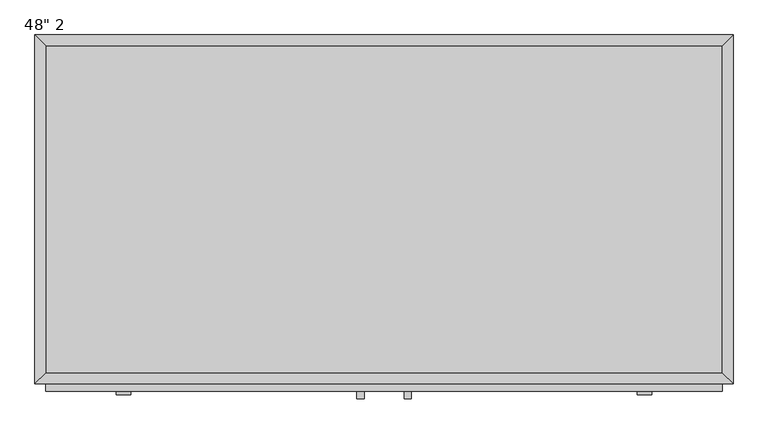
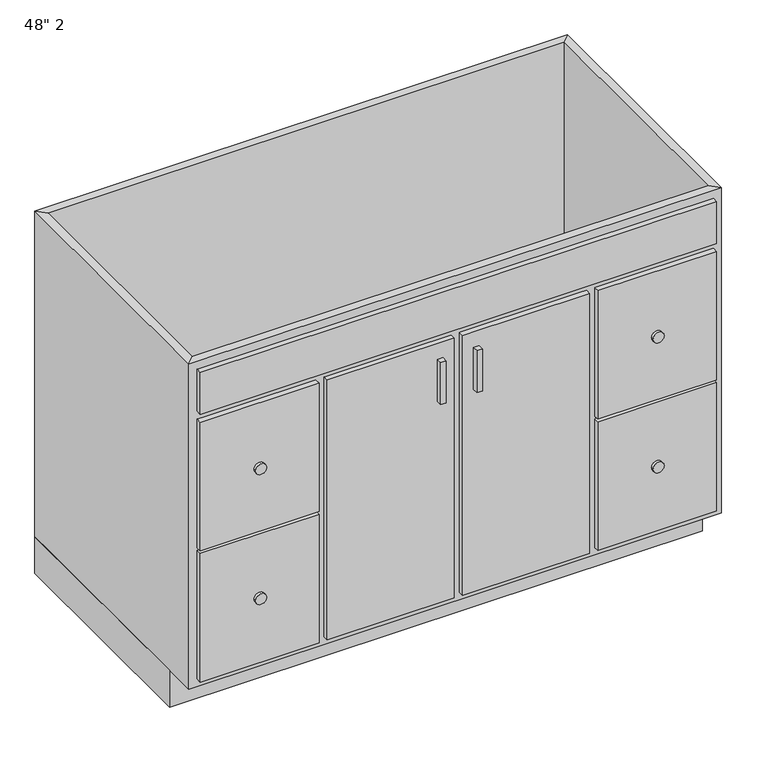
"""IFC4 building model written with IfcOpenShell, lengths in millimetres: furniture geometry."""

from ifc_helpers import new_model, si_unit, point, frame, frame_2d, origin, origin_with_axes, place, context, project, spatial, polyline, circle_curve, trimmed, segment, composite_curve, outline, extrude, faceted_brep, source, transform, mapped, element, save


def furniture_3428e43d(model_context):
    return source(origin(), model_context, "Body", "SolidModel", [
        extrude(outline(polyline([(700.44496, 0.0), (700.44496, -533.4), (-518.75504, -533.4), (-518.75504, 0.0), (700.44496, 0.0)])), origin_with_axes(), (0.0, 0.0, 1.0), 88.9),
        faceted_brep([(681.39496, -590.55, 876.3), (681.39496, -590.55, 88.9), (-499.70504, -590.55, 88.9), (-499.70504, -590.55, 876.3), (700.44496, -609.6, 876.3), (-518.75504, -609.6, 876.3), (700.44496, -609.6, 88.9), (-518.75504, -609.6, 88.9), (-499.70504, -19.05, 88.9), (-499.70504, -19.05, 876.3), (-518.75504, 0.0, 876.3), (-518.75504, 0.0, 88.9), (681.39496, -19.05, 88.9), (681.39496, -19.05, 876.3), (700.44496, 0.0, 876.3), (700.44496, 0.0, 88.9)], [[[0, 1, 2, 3]], [[4, 0, 3, 5]], [[6, 4, 5, 7]], [[1, 6, 7, 2]], [[3, 2, 8, 9]], [[5, 3, 9, 10]], [[7, 5, 10, 11]], [[2, 7, 11, 8]], [[9, 8, 12, 13]], [[10, 9, 13, 14]], [[11, 10, 14, 15]], [[8, 11, 15, 12]], [[13, 12, 1, 0]], [[14, 13, 0, 4]], [[15, 14, 4, 6]], [[12, 15, 6, 1]]]),
        extrude(outline(polyline([(681.39496, -19.05), (681.39496, -590.55), (-499.70504, -590.55), (-499.70504, -19.05), (681.39496, -19.05)])), frame((0.0, 0.0, 88.9), z_axis=(0.0, 0.0, 1.0), x_axis=(1.0, 0.0, 0.0)), (0.0, 0.0, 1.0), 19.05),
        extrude(outline(composite_curve([segment(trimmed(circle_curve(frame_2d((265.1125, 545.66371)), 12.7), [point((265.1125, 532.96371))], [point((265.1125, 558.36371))], False, "CARTESIAN"), True, "CONTINUOUS"), segment(trimmed(circle_curve(frame_2d((265.1125, 545.66371)), 12.7), [point((265.1125, 558.36371))], [point((265.1125, 532.96371))], False, "CARTESIAN"), True, "CONTINUOUS")], self_intersect=False)), frame((0.0, -628.65, 0.0), z_axis=(0.0, 1.0, 0.0), x_axis=(0.0, 0.0, 1.0)), (0.0, 0.0, 1.0), 6.35),
        extrude(outline(composite_curve([segment(trimmed(circle_curve(frame_2d((579.4375, 545.66371)), 12.7), [point((579.4375, 532.96371))], [point((579.4375, 558.36371))], False, "CARTESIAN"), True, "CONTINUOUS"), segment(trimmed(circle_curve(frame_2d((579.4375, 545.66371)), 12.7), [point((579.4375, 558.36371))], [point((579.4375, 532.96371))], False, "CARTESIAN"), True, "CONTINUOUS")], self_intersect=False)), frame((0.0, -628.65, 0.0), z_axis=(0.0, 1.0, 0.0), x_axis=(0.0, 0.0, 1.0)), (0.0, 0.0, 1.0), 6.35),
        extrude(outline(composite_curve([segment(trimmed(circle_curve(frame_2d((579.4375, -363.97379)), 12.7), [point((579.4375, -376.67379))], [point((579.4375, -351.27379))], False, "CARTESIAN"), True, "CONTINUOUS"), segment(trimmed(circle_curve(frame_2d((579.4375, -363.97379)), 12.7), [point((579.4375, -351.27379))], [point((579.4375, -376.67379))], False, "CARTESIAN"), True, "CONTINUOUS")], self_intersect=False)), frame((0.0, -628.65, 0.0), z_axis=(0.0, 1.0, 0.0), x_axis=(0.0, 0.0, 1.0)), (0.0, 0.0, 1.0), 6.35),
        extrude(outline(composite_curve([segment(trimmed(circle_curve(frame_2d((265.1125, -363.97379)), 12.7), [point((265.1125, -376.67379))], [point((265.1125, -351.27379))], False, "CARTESIAN"), True, "CONTINUOUS"), segment(trimmed(circle_curve(frame_2d((265.1125, -363.97379)), 12.7), [point((265.1125, -351.27379))], [point((265.1125, -376.67379))], False, "CARTESIAN"), True, "CONTINUOUS")], self_intersect=False)), frame((0.0, -628.65, 0.0), z_axis=(0.0, 1.0, 0.0), x_axis=(0.0, 0.0, 1.0)), (0.0, 0.0, 1.0), 6.35),
        extrude(outline(polyline([(55.91996, -635.0), (43.21996, -635.0), (43.21996, -622.3), (55.91996, -622.3), (55.91996, -635.0)])), frame((0.0, 0.0, 596.9), z_axis=(0.0, 0.0, 1.0), x_axis=(1.0, 0.0, 0.0)), (0.0, 0.0, 1.0), 101.6),
        extrude(outline(polyline([(138.46996, -635.0), (125.76996, -635.0), (125.76996, -622.3), (138.46996, -622.3), (138.46996, -635.0)])), frame((0.0, 0.0, 596.9), z_axis=(0.0, 0.0, 1.0), x_axis=(1.0, 0.0, 0.0)), (0.0, 0.0, 1.0), 101.6),
        extrude(outline(polyline([(681.39496, -622.3), (-499.70504, -622.3), (-499.70504, -609.6), (681.39496, -609.6), (681.39496, -622.3)])), frame((0.0, 0.0, 755.65), z_axis=(0.0, 0.0, 1.0), x_axis=(1.0, 0.0, 0.0)), (0.0, 0.0, 1.0), 101.6),
        extrude(outline(polyline([(681.39496, -622.3), (409.93246, -622.3), (409.93246, -609.6), (681.39496, -609.6), (681.39496, -622.3)])), frame((0.0, 0.0, 425.45), z_axis=(0.0, 0.0, 1.0), x_axis=(1.0, 0.0, 0.0)), (0.0, 0.0, 1.0), 311.15),
        extrude(outline(polyline([(681.39496, -622.3), (409.93246, -622.3), (409.93246, -609.6), (681.39496, -609.6), (681.39496, -622.3)])), frame((0.0, 0.0, 107.95), z_axis=(0.0, 0.0, 1.0), x_axis=(1.0, 0.0, 0.0)), (0.0, 0.0, 1.0), 311.15),
        extrude(outline(polyline([(-228.24254, -622.3), (-499.70504, -622.3), (-499.70504, -609.6), (-228.24254, -609.6), (-228.24254, -622.3)])), frame((0.0, 0.0, 425.45), z_axis=(0.0, 0.0, 1.0), x_axis=(1.0, 0.0, 0.0)), (0.0, 0.0, 1.0), 311.15),
        extrude(outline(polyline([(-228.24254, -622.3), (-499.70504, -622.3), (-499.70504, -609.6), (-228.24254, -609.6), (-228.24254, -622.3)])), frame((0.0, 0.0, 107.95), z_axis=(0.0, 0.0, 1.0), x_axis=(1.0, 0.0, 0.0)), (0.0, 0.0, 1.0), 311.15),
        extrude(outline(polyline([(81.31996, -622.3), (-209.19254, -622.3), (-209.19254, -609.6), (81.31996, -609.6), (81.31996, -622.3)])), frame((0.0, 0.0, 107.95), z_axis=(0.0, 0.0, 1.0), x_axis=(1.0, 0.0, 0.0)), (0.0, 0.0, 1.0), 628.65),
        extrude(outline(polyline([(390.88246, -622.3), (100.36996, -622.3), (100.36996, -609.6), (390.88246, -609.6), (390.88246, -622.3)])), frame((0.0, 0.0, 107.95), z_axis=(0.0, 0.0, 1.0), x_axis=(1.0, 0.0, 0.0)), (0.0, 0.0, 1.0), 628.65),
    ])


if __name__ == "__main__":
    model = new_model("IFC4")
    model_context = context("Model", 3, world=origin())
    ifc_project = project(units=[si_unit("LENGTHUNIT", "METRE", prefix="MILLI")], contexts=[model_context])
    site = spatial("IfcSite", under=ifc_project)
    building = spatial("IfcBuilding", under=site)
    placement = place(None, origin())
    furniture_shape = furniture_3428e43d(model_context)
    element("IfcFurniture", 1, ObjectType="48\" 2", at=placement, inside=building, context=model_context, shape_type="MappedRepresentation", body=[
        mapped(furniture_shape, transform((0.0, 0.0, 0.0), x_axis=(1.0, 0.0, 0.0), y_axis=(0.0, 1.0, 0.0), z_axis=(0.0, 0.0, 1.0))),
    ])
    save(model, "model.ifc")

# Revit data of these elements
# Type "48\" 2"
#   Assembly Code = "C1030410"
#   Depth = 2' - 0"
#   Height = 2' - 10 1/2"
#   Toe Depth = 0' - 3"
#   Toe Height = 0' - 3 1/2"
#   Width = 4' - 0"
#   Cabinet Material = none
#   Door/Drawer Material = none
#   Handle Material = Cabinets - Handles
#   Default Elevation = 0
# Element 1 (IfcFurniture, "48\" 2")
#   Materials on its faces: "Cabinet", "Cabinets - Handles", "Cabinets"
# Materials
#   "Cabinets - Handles": colour RGB 57 57 57, transparency 0
#   "Cabinet": colour RGB 204 122 2, transparency 0
#   "Cabinets": colour RGB 249 249 249, transparency 0
